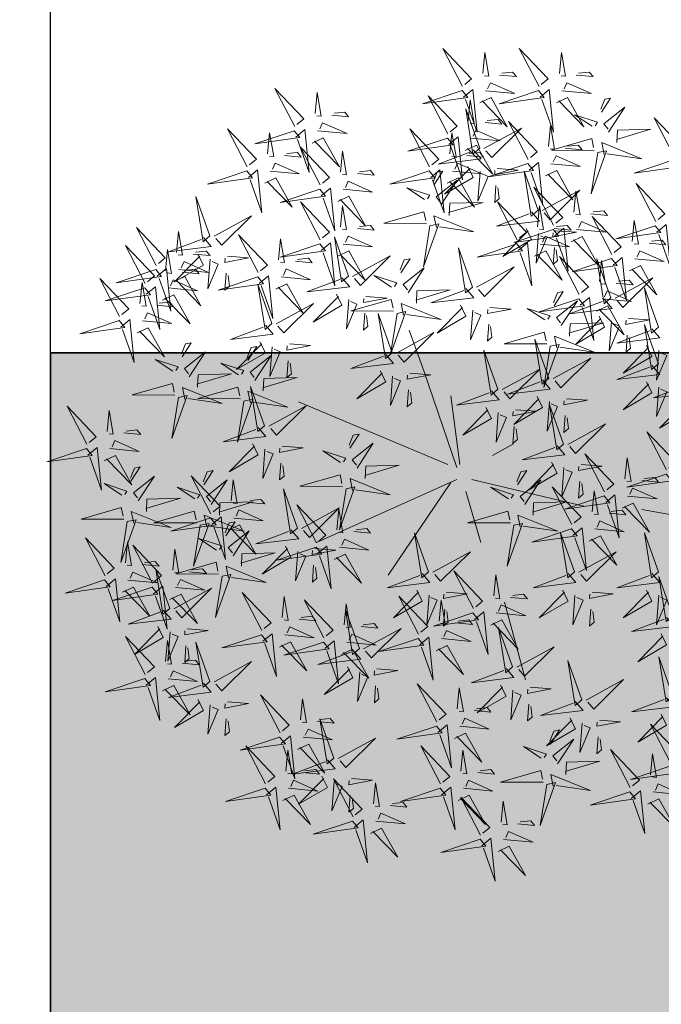
# Model space of a CAD drawing. Units: inches. Extents: x 1704 to 6393, y -157 to 1172.
# Tile 70 of 122: x 1897 to 1920, y 1010 to 1045. Entities that reach past the tile are written whole.
import ezdxf

# ---------------------------------------------------------------- set-up
doc = ezdxf.new("R2010")
doc.units = ezdxf.units.IN
doc.header["$MEASUREMENT"] = 0
for name, color, linetype, lineweight in [('A-ANNO-DIMS', 7, 'Continuous', 13), ('C-PROP', 7, 'Continuous', 35), ('L-shrub', 74, 'Continuous', 18), ('L-tree', 102, 'Continuous', 18)]:
    doc.layers.add(name, color=color, linetype=linetype, lineweight=lineweight)
doc.layers.add('L-HRDS-PATT', color=9, linetype='Continuous', lineweight=13, true_color=0xc5c1ba)
doc.styles.get("Standard").update_dxf_attribs({"font": 'arial.ttf'})
doc.dimstyles.get("Standard").update_dxf_attribs({"dimtxt": 6, "dimasz": 2, "dimexe": 0.18, "dimexo": 0.0625, "dimgap": 0.09, "dimtad": 0, "dimtih": 1, "dimtoh": 1, "dimdec": 1, "dimzin": 0, "dimdsep": 46, "dimlunit": 3, "dimtxsty": 'Standard', "dimblk": 'ARCHTICK', "dimcen": 0.09, "dimadec": 0, "dimazin": 0, "dimtfac": 1, "dimtdec": 1, "dimtofl": 0, "dimtmove": 0, "dimatfit": 3, "dimfxl": 1, "dimtolj": 1, "dimtzin": 0, "dimarcsym": 0})

# ---------------------------------------------------------------- blocks, each defined once
blk = doc.blocks.new('bamboo')
blk.add_line((390, 162.3), (546.4, 218.1))
at = {"layer": 'L-shrub'}
for p, q in [((43.5, 73), (278.2, 631.2)), ((-12.4, 39.5), (-247.1, 564.2)), ((-23.6, 61.9), (-370, 296.3)), ((32.3, 39.5), (390, 162.3)), ((43.5, 28.4), (300.5, 61.9)), ((-57.1, 6), (-247.1, -49.8)), ((-12.4, -16.3), (-113, -440.5)), ((77, -94.4), (121.7, -172.6)), ((-470.6, -139.1), (-761.2, -217.2)), ((-124.2, -652.6), (-157.7, -842.3))]:
    blk.add_line(p, q, dxfattribs=at)
for points in [[(103.7, 1424.7), (54.4, 1572.3), (77.9, 1403.4), (103.7, 1424.7)], [(-387.8, 1356.5), (-437.1, 1504.1), (-413.6, 1335.2), (-387.8, 1356.5)], [(119.4, 1423.2), (261.4, 1496.7), (147.9, 1388.7), (126.6, 1414.5)], [(-160.7, 1284.9), (-160, 1444.8), (-116.9, 1294.1), (-149.7, 1287.2)], [(581.6, 1302), (532.2, 1449.6), (555.7, 1280.7), (581.6, 1302)], [(-372, 1355), (-230.1, 1428.5), (-343.6, 1320.5), (-364.9, 1346.4)], [(79.4, 1419.1), (107.8, 1384.6), (-52.4, 1368.4), (70.8, 1412)], [(597.3, 1300.4), (739.2, 1374), (625.7, 1265.9), (604.4, 1291.8)], [(-756.4, 1206.5), (-805.8, 1354.1), (-782.2, 1185.2), (-756.4, 1206.5)], [(-412.1, 1350.9), (-383.7, 1316.4), (-543.9, 1300.2), (-420.7, 1343.8)], [(-415.1, 1179.2), (-464.4, 1326.8), (-440.9, 1157.9), (-415.1, 1179.2)], [(-70.9, 1292.4), (-27.7, 1358.5), (-55.4, 1272.9), (-68.6, 1281.5)], [(57.7, 1357.7), (77.5, 1316.1), (-31.5, 1255.3), (64.8, 1349.1)], [(103.3, 1337.4), (92.8, 1227.4), (133.3, 1318.7), (110.4, 1328.8)], [(167.7, 1347.1), (246.3, 1339.5), (157.6, 1324.2), (159.1, 1340)], [(704.4, 1206.5), (655.1, 1354.1), (678.6, 1185.2), (704.4, 1206.5)], [(-433.8, 1289.5), (-414, 1248), (-523, 1187.1), (-426.7, 1280.9)], [(-169.3, 1271.7), (-323, 1296.4), (-162.4, 1238.9), (-169.3, 1271.7)], [(557.2, 1296.4), (585.7, 1261.9), (425.4, 1245.7), (548.6, 1289.3)], [(772.7, 1165.6), (723.3, 1313.2), (746.9, 1144.3), (772.7, 1165.6)], [(-740.7, 1205), (-598.8, 1278.5), (-712.2, 1170.5), (-733.6, 1196.4)], [(-500.1, 1137.3), (-534, 1108.2), (-553.5, 1268), (-507.4, 1145.8)], [(-388.2, 1269.3), (-398.7, 1159.2), (-358.2, 1250.5), (-381.1, 1260.6)], [(-323.8, 1278.9), (-245.2, 1271.3), (-333.9, 1256.1), (-332.4, 1271.8)], [(-175.7, 1247.6), (-131.9, 1256.8), (-191.9, 1107.3), (-173.4, 1236.6)], [(-18, 1257.9), (35, 1223.4), (30.4, 1245.3), (-7, 1260.2)], [(161.7, 1284.2), (155.7, 1221.3), (172.9, 1235.5), (168.8, 1275.6)], [(303.5, 1094), (304.2, 1253.9), (347.3, 1103.2), (314.4, 1096.3)], [(720.2, 1205), (862.1, 1278.5), (748.6, 1170.5), (727.3, 1196.4)], [(-561.9, 1157.8), (-603.1, 1137.1), (-666.2, 1244.8), (-570.4, 1150.5)], [(-399.4, 1177.7), (-257.4, 1251.3), (-370.9, 1143.2), (-392.2, 1169.1)], [(-329.8, 1216), (-335.8, 1153.1), (-318.6, 1167.3), (-322.7, 1207.4)], [(-92.2, 1230.9), (0.4, 1170.5), (-61.7, 1248.7), (-81.3, 1233.2)], [(535.5, 1235), (555.3, 1193.4), (446.4, 1132.5), (542.6, 1226.4)], [(581.2, 1214.7), (570.7, 1104.6), (611.1, 1195.9), (588.3, 1206.1)], [(645.6, 1224.3), (724.2, 1216.7), (635.4, 1201.5), (637, 1217.2)], [(788.4, 1164.1), (930.3, 1237.6), (816.9, 1129.6), (795.5, 1155.5)], [(-780.7, 1200.9), (-752.3, 1166.4), (-912.5, 1150.2), (-789.3, 1193.8)], [(-131.4, 1199.8), (-85.3, 1198.1), (-81.9, 1073.4), (-120.4, 1202.1)], [(680.1, 1200.9), (708.6, 1166.4), (548.3, 1150.2), (671.5, 1193.8)], [(-439.4, 1173.7), (-411, 1139.2), (-571.2, 1122.9), (-448, 1166.6)], [(-494, 1113.1), (-347.5, 1165.5), (-515.9, 1138.5), (-494, 1113.1)], [(-174.3, 1012.2), (-173.7, 1172.1), (-130.6, 1021.4), (-163.4, 1014.5)], [(393.3, 1101.5), (436.5, 1167.6), (408.8, 1082), (395.6, 1090.6)], [(748.4, 1160), (776.8, 1125.5), (616.6, 1109.3), (739.8, 1152.9)], [(639.6, 1161.5), (633.5, 1098.6), (650.8, 1112.8), (646.7, 1152.8)], [(-802.5, 1139.6), (-782.6, 1098), (-891.6, 1037.1), (-795.3, 1130.9)], [(-773.2, 987.3), (-807.1, 958.2), (-826.6, 1118), (-780.4, 995.8)], [(-756.8, 1119.3), (-767.3, 1009.2), (-726.8, 1100.5), (-749.7, 1110.6)], [(-692.4, 1128.9), (-613.8, 1121.3), (-702.5, 1106.1), (-701, 1121.8)], [(-581.3, 1111.7), (-691.5, 1120), (-599.4, 1081.4), (-589.8, 1104.4)], [(-461.1, 1112.3), (-441.3, 1070.7), (-550.3, 1009.8), (-454, 1103.7)], [(-155.7, 961.1), (-205, 1108.7), (-181.5, 939.8), (-155.7, 961.1)], [(294.9, 1080.8), (141.2, 1105.5), (301.8, 1048), (294.9, 1080.8)], [(658.4, 1139.6), (678.2, 1098), (569.2, 1037.1), (665.5, 1130.9)], [(704, 1119.3), (693.5, 1009.2), (734, 1100.5), (711.2, 1110.6)], [(768.4, 1128.9), (847.1, 1121.3), (758.3, 1106.1), (759.8, 1121.8)], [(892.5, 987.3), (858.6, 958.2), (839.1, 1118), (885.2, 995.8)], [(-835, 1007.8), (-876.2, 987.1), (-939.2, 1094.8), (-843.4, 1000.5)], [(-495.2, 1097.3), (-418.8, 957), (-529.1, 1068.2), (-503.7, 1090.1)], [(-415.5, 1092), (-426, 981.9), (-385.5, 1073.2), (-408.4, 1083.4)], [(-365.5, 930.4), (-364.8, 1090.2), (-321.7, 939.6), (-354.5, 932.7)], [(-351.1, 1101.6), (-272.5, 1094), (-361.2, 1078.8), (-359.7, 1094.5)], [(-84.5, 1019.7), (-41.3, 1085.8), (-69, 1000.1), (-82.2, 1008.8)], [(446.2, 1067), (499.2, 1032.5), (494.6, 1054.4), (457.2, 1069.3)], [(726.6, 1098.6), (746.5, 1057), (637.5, 996.2), (733.8, 1090)], [(830.7, 1007.8), (789.5, 987.1), (726.4, 1094.8), (822.2, 1000.5)], [(772.3, 1078.4), (761.8, 968.3), (802.3, 1059.6), (779.4, 1069.7)], [(836.7, 1088), (915.3, 1080.4), (826.6, 1065.2), (828.1, 1080.9)], [(-698.4, 1066), (-704.4, 1003.1), (-687.2, 1017.3), (-691.3, 1057.4)], [(-633.3, 1052.3), (-696.3, 1057), (-681.8, 1040.1), (-641.8, 1045)], [(-570.3, 1047.5), (-576.3, 968.8), (-593.4, 1057.2), (-577.6, 1056)], [(-357.1, 1038.7), (-363.1, 975.8), (-345.9, 990), (-350, 1030.1)], [(-140, 959.5), (2, 1033.1), (-111.5, 925), (-132.8, 950.9)], [(288.5, 1056.7), (332.3, 1065.9), (272.3, 916.4), (290.8, 1045.7)], [(372, 1040), (464.6, 979.6), (402.5, 1057.8), (382.9, 1042.3)], [(762.4, 1066), (756.4, 1003.1), (773.6, 1017.3), (769.5, 1057.4)], [(-767.1, 963.1), (-620.5, 1015.5), (-788.9, 988.5), (-767.1, 963.1)], [(-183, 999), (-336.7, 1023.7), (-176.1, 966.2), (-183, 999)], [(-275.7, 937.9), (-232.5, 1004), (-260.1, 918.3), (-273.4, 927)], [(289.9, 848.6), (290.5, 1008.4), (333.6, 857.8), (300.8, 850.9)], [(332.8, 1008.9), (378.9, 1007.2), (382.3, 882.5), (343.8, 1011.2)], [(830.7, 1025.1), (824.7, 962.2), (841.9, 976.4), (837.8, 1016.5)], [(898.5, 963.1), (1045.1, 1015.5), (876.7, 988.5), (898.5, 963.1)], [(-854.3, 961.7), (-964.6, 970), (-872.5, 931.4), (-862.8, 954.4)], [(-189.3, 974.8), (-145.6, 984), (-205.5, 834.6), (-187, 963.9)], [(-105.9, 958.2), (-13.2, 897.8), (-75.4, 976), (-94.9, 960.5)], [(-31.6, 985.2), (21.3, 950.7), (16.7, 972.5), (-20.7, 987.5)], [(811.3, 961.7), (701, 970), (793.1, 931.4), (802.8, 954.4)], [(1141.3, 824.7), (1092, 972.3), (1115.5, 803.4), (1141.3, 824.7)], [(-768.3, 947.3), (-691.9, 807), (-802.2, 918.2), (-776.8, 940.1)], [(-374.1, 917.2), (-527.8, 941.9), (-367.2, 884.4), (-374.1, 917.2)], [(-180, 955.5), (-151.6, 921), (-311.8, 904.8), (-188.6, 948.4)], [(-145, 927.1), (-99, 925.4), (-95.6, 800.6), (-134.1, 929.4)], [(379.6, 856.1), (422.9, 922.2), (395.2, 836.5), (381.9, 845.1)], [(745.4, 783.8), (696, 931.4), (719.6, 762.5), (745.4, 783.8)], [(897.3, 947.3), (973.8, 807), (863.4, 918.2), (888.9, 940.1)], [(-1166, 756.5), (-1215.3, 904.1), (-1191.8, 735.2), (-1166, 756.5)], [(-906.4, 902.3), (-969.4, 907), (-954.8, 890.1), (-914.9, 895)], [(-843.4, 897.5), (-849.4, 818.8), (-866.4, 907.2), (-850.7, 906)], [(-592.6, 770.2), (-641.9, 917.8), (-618.4, 748.9), (-592.6, 770.2)], [(-380.5, 893), (-336.7, 902.2), (-396.6, 752.7), (-378.2, 882.1)], [(-297, 876.4), (-204.4, 816), (-266.5, 894.2), (-286.1, 878.7)], [(-201.7, 894.1), (-181.9, 852.5), (-290.9, 791.6), (-194.6, 885.5)], [(-222.7, 903.4), (-169.8, 868.9), (-174.4, 890.7), (-211.8, 905.7)], [(-91.7, 883.5), (-13.1, 875.8), (-101.8, 860.6), (-100.3, 876.4)], [(120.7, 803.3), (79.5, 782.6), (16.5, 890.3), (112.2, 796)], [(182.5, 782.8), (148.6, 753.6), (129.1, 913.5), (175.2, 791.2)], [(564.8, 755.5), (530.9, 726.4), (511.4, 886.2), (557.5, 764)], [(759.2, 902.3), (696.2, 907), (710.8, 890.1), (750.8, 895)], [(822.2, 897.5), (816.2, 818.8), (799.2, 907.2), (815, 906)], [(1157.1, 823.2), (1299, 896.7), (1185.5, 788.7), (1164.2, 814.6)], [(-974.8, 702), (-1024.2, 849.6), (-1000.7, 680.7), (-974.8, 702)], [(-336.2, 845.3), (-290.1, 843.6), (-286.7, 718.8), (-325.2, 847.6)], [(-156.1, 873.8), (-166.6, 763.7), (-126.1, 855), (-149, 865.2)], [(281.2, 835.4), (127.5, 860.1), (288.1, 802.6), (281.2, 835.4)], [(503, 776), (461.8, 755.3), (398.7, 863), (494.5, 768.7)], [(761.1, 782.3), (903, 855.8), (789.6, 747.8), (768.2, 773.7)], [(-1150.2, 755), (-1008.3, 828.6), (-1121.8, 720.5), (-1143.1, 746.4)], [(-576.8, 768.6), (-434.9, 842.2), (-548.4, 734.1), (-569.7, 760)], [(-97.7, 820.6), (-103.7, 757.7), (-86.5, 771.9), (-90.6, 811.9)], [(188.6, 758.6), (335.2, 810.9), (166.8, 784), (188.6, 758.6)], [(274.9, 811.2), (318.6, 820.4), (258.7, 670.9), (277.2, 800.3)], [(358.3, 794.5), (451, 734.2), (388.8, 812.4), (369.3, 796.8)], [(432.6, 821.6), (485.5, 787.1), (480.9, 808.9), (443.5, 823.9)], [(1117, 819.1), (1145.4, 784.6), (985.2, 768.4), (1108.4, 812)], [(-959.1, 700.5), (-817.2, 774), (-930.7, 666), (-952, 691.8)], [(-199.8, 660.1), (-233.7, 630.9), (-253.2, 790.8), (-207, 668.5)], [(570.9, 731.3), (717.4, 783.7), (549, 756.7), (570.9, 731.3)], [(721.1, 778.2), (749.5, 743.7), (589.3, 727.5), (712.5, 771.1)], [(1291.5, 647.4), (1242.1, 795), (1265.7, 626.1), (1291.5, 647.4)], [(-1190.3, 750.9), (-1161.9, 716.5), (-1322.1, 700.2), (-1198.9, 743.8)], [(-616.9, 764.6), (-588.5, 730.1), (-748.7, 713.9), (-625.5, 757.5)], [(-261.6, 680.5), (-302.7, 659.9), (-365.8, 767.6), (-270, 673.2)], [(101.4, 757.2), (-8.9, 765.5), (83.2, 726.9), (92.9, 749.9)], [(187.4, 742.8), (263.8, 602.4), (153.5, 713.7), (178.9, 735.5)], [(319.2, 763.5), (365.2, 761.8), (368.6, 637), (330.1, 765.8)], [(483.6, 729.9), (373.4, 738.2), (465.5, 699.6), (475.2, 722.6)], [(1095.3, 757.7), (1115.1, 716.2), (1006.1, 655.3), (1102.4, 749.1)], [(1140.9, 737.5), (1130.4, 627.4), (1170.9, 718.7), (1148, 728.8)], [(1205.3, 747.1), (1283.9, 739.5), (1195.2, 724.3), (1196.7, 740)], [(-638.6, 703.2), (-618.8, 661.6), (-727.8, 600.7), (-631.5, 694.6)], [(-264.9, 565.6), (-314.3, 713.2), (-290.7, 544.3), (-264.9, 565.6)], [(49.3, 697.7), (-13.7, 702.5), (0.8, 685.5), (40.8, 690.4)], [(112.3, 693), (106.3, 614.2), (89.3, 702.6), (105, 701.5)], [(569.7, 715.5), (646.1, 575.2), (535.8, 686.4), (561.2, 708.3)], [(699.3, 716.8), (719.2, 675.2), (610.2, 614.4), (706.4, 708.2)], [(809.4, 706.2), (888, 698.6), (799.3, 683.4), (800.8, 699.1)], [(868.3, 552), (818.9, 699.6), (842.4, 530.7), (868.3, 552)], [(1073.1, 552), (1023.7, 699.6), (1047.2, 530.7), (1073.1, 552)], [(1307.2, 645.9), (1449.1, 719.5), (1335.7, 611.4), (1314.3, 637.3)], [(-1212, 689.6), (-1192.2, 648), (-1301.2, 587.1), (-1204.9, 680.9)], [(-1166.4, 669.3), (-1176.9, 559.2), (-1136.4, 650.5), (-1159.3, 660.7)], [(-999.2, 696.4), (-970.7, 661.9), (-1131, 645.7), (-1007.8, 689.3)], [(-1102, 678.9), (-1023.4, 671.3), (-1112.1, 656.1), (-1110.6, 671.8)], [(-619.9, 538.4), (-669.2, 686), (-645.7, 517), (-619.9, 538.4)], [(-593, 682.9), (-603.5, 572.8), (-563, 664.1), (-585.9, 674.3)], [(-528.6, 692.6), (-450, 684.9), (-538.7, 669.7), (-537.2, 685.5)], [(-193.7, 635.8), (-47.1, 688.2), (-215.5, 661.2), (-193.7, 635.8)], [(431.6, 670.5), (368.6, 675.2), (383.1, 658.2), (423.1, 663.2)], [(494.6, 665.7), (488.6, 587), (471.6, 675.4), (487.3, 674.2)], [(745, 696.6), (734.5, 586.5), (774.9, 677.8), (752.1, 687.9)], [(1199.3, 684.2), (1193.3, 621.3), (1210.5, 635.5), (1206.4, 675.6)], [(-1121.7, 544.2), (-1162.9, 523.5), (-1225.9, 631.2), (-1130.2, 536.9)], [(-1059.9, 523.7), (-1093.8, 494.6), (-1113.3, 654.4), (-1067.1, 532.2)], [(-1020.9, 635), (-1001.1, 593.4), (-1110, 532.6), (-1013.8, 626.4)], [(-534.6, 629.7), (-540.6, 566.8), (-523.4, 581), (-527.5, 621)], [(-280.9, 634.5), (-391.2, 642.7), (-299.1, 604.1), (-289.4, 627.2)], [(-249.2, 564.1), (-107.3, 637.7), (-220.7, 529.6), (-242.1, 555.5)], [(-37.8, 466.8), (-37.2, 626.6), (5.9, 476), (-26.9, 469.1)], [(803.4, 643.3), (797.4, 580.4), (814.6, 594.6), (810.5, 634.7)], [(1267.2, 641.9), (1295.6, 607.4), (1135.4, 591.1), (1258.6, 634.8)], [(-1108, 616), (-1114, 553.1), (-1096.8, 567.3), (-1100.9, 607.4)], [(-975.2, 614.7), (-985.8, 504.7), (-945.3, 596), (-968.1, 606.1)], [(-910.8, 624.4), (-832.2, 616.8), (-921, 601.5), (-919.5, 617.3)], [(-604.1, 536.8), (-462.2, 610.4), (-575.7, 502.3), (-597, 528.2)], [(-194.9, 620.1), (-118.4, 479.7), (-228.8, 591), (-203.4, 612.8)], [(742.3, 469.2), (708.4, 440), (688.9, 599.9), (735, 477.6)], [(884, 550.5), (1025.9, 624), (912.4, 516), (891.1, 541.8)], [(1088.8, 550.5), (1230.7, 624), (1117.2, 516), (1095.9, 541.8)], [(-1288.8, 429.3), (-1338.2, 576.9), (-1314.7, 408), (-1288.8, 429.3)], [(-916.9, 561.5), (-922.9, 498.6), (-905.6, 512.8), (-909.7, 552.9)], [(-650.3, 428.2), (-684.2, 399.1), (-703.7, 559), (-657.6, 436.7)], [(-289.2, 560), (-260.8, 525.6), (-421, 509.3), (-297.8, 552.9)], [(-333, 575), (-396, 579.7), (-381.4, 562.8), (-341.5, 567.7)], [(-270, 570.3), (-276, 491.5), (-293, 579.9), (-277.2, 578.7)], [(680.5, 489.6), (639.3, 469), (576.2, 576.7), (672, 482.3)], [(1245.4, 580.5), (1265.3, 538.9), (1156.3, 478), (1252.6, 571.9)], [(1291.1, 560.2), (1280.6, 450.1), (1321.1, 541.4), (1298.2, 551.6)], [(1355.5, 569.8), (1434.1, 562.2), (1345.4, 547), (1346.9, 562.7)], [(-1053.8, 499.5), (-907.2, 551.9), (-1075.6, 524.9), (-1053.8, 499.5)], [(-712.1, 448.7), (-753.3, 428.1), (-816.4, 535.7), (-720.6, 441.4)], [(-644.2, 532.8), (-615.8, 498.3), (-776, 482), (-652.8, 525.7)], [(52, 474.3), (95.2, 540.4), (67.5, 454.7), (54.3, 463.3)], [(843.9, 546.4), (872.4, 511.9), (712.1, 495.7), (835.3, 539.3)], [(1048.7, 546.4), (1077.2, 511.9), (916.9, 495.7), (1040.1, 539.3)], [(-1273.1, 427.7), (-1131.2, 501.3), (-1244.7, 393.3), (-1266, 419.1)], [(-1141, 498.1), (-1251.3, 506.4), (-1159.2, 467.8), (-1149.5, 490.8)], [(-1055, 483.7), (-978.6, 343.4), (-1088.9, 454.6), (-1063.5, 476.4)], [(-311, 498.7), (-291.1, 457.1), (-400.1, 396.2), (-303.9, 490)], [(-200.9, 488), (-122.3, 480.4), (-211, 465.2), (-209.5, 480.9)], [(748.4, 444.9), (894.9, 497.3), (726.5, 470.3), (748.4, 444.9)], [(822.2, 485), (842, 443.4), (733.1, 382.6), (829.3, 476.4)], [(1027, 485), (1046.8, 443.4), (937.9, 382.6), (1034.1, 476.4)], [(1349.5, 506.9), (1343.5, 444), (1360.7, 458.2), (1356.6, 498.3)], [(-1193.1, 438.6), (-1256.1, 443.4), (-1241.5, 426.4), (-1201.6, 431.4)], [(-1130.1, 433.9), (-1136.1, 355.2), (-1153.1, 443.6), (-1137.4, 442.4)], [(-665.9, 471.4), (-646.1, 429.8), (-755.1, 368.9), (-658.8, 462.8)], [(-644.2, 404), (-497.6, 456.4), (-666, 429.4), (-644.2, 404)], [(-620.3, 451.1), (-630.8, 341), (-590.3, 432.3), (-613.2, 442.5)], [(-555.9, 460.7), (-477.3, 453.1), (-566, 437.9), (-564.5, 453.6)], [(-265.3, 478.4), (-275.8, 368.3), (-235.4, 459.6), (-258.2, 469.8)], [(-46.5, 453.6), (-200.1, 478.3), (-39.6, 420.8), (-46.5, 453.6)], [(104.9, 439.8), (157.9, 405.3), (153.3, 427.1), (115.9, 442.1)], [(661.1, 443.6), (550.9, 451.8), (643, 413.2), (652.6, 436.3)], [(867.9, 464.7), (857.4, 354.7), (897.8, 446), (875, 456.1)], [(932.3, 474.4), (1010.9, 466.8), (922.2, 451.6), (923.7, 467.3)], [(1072.7, 464.7), (1062.1, 354.7), (1102.6, 446), (1079.8, 456.1)], [(1137.1, 474.4), (1215.7, 466.8), (1126.9, 451.6), (1128.4, 467.3)], [(-1313.2, 423.7), (-1284.7, 389.2), (-1445, 373), (-1321.8, 416.6)], [(-731.5, 402.7), (-841.7, 410.9), (-749.6, 372.3), (-739.9, 395.4)], [(-206.9, 425.1), (-212.9, 362.2), (-195.7, 376.4), (-199.8, 416.5)], [(-52.8, 429.4), (-9, 438.6), (-69, 289.1), (-50.5, 418.5)], [(30.7, 412.7), (123.3, 352.4), (61.2, 430.6), (41.6, 415)], [(393.8, 326), (352.6, 305.3), (289.5, 413), (385.3, 318.7)], [(455.6, 305.5), (421.7, 276.4), (402.2, 436.3), (448.3, 314)], [(617.5, 275.9), (618.2, 435.7), (661.3, 285.1), (628.5, 278.2)], [(747.2, 429.2), (823.6, 288.8), (713.3, 400), (738.7, 421.9)], [(926.3, 411.5), (920.3, 348.6), (937.5, 362.8), (933.4, 402.9)], [(1131.1, 411.5), (1125, 348.6), (1142.3, 362.8), (1138.2, 402.9)], [(-645.4, 388.3), (-569, 247.9), (-679.3, 359.1), (-653.9, 381)], [(-561.9, 397.8), (-567.9, 334.9), (-550.7, 349.1), (-554.8, 389.2)], [(-8.5, 381.7), (37.5, 380), (40.9, 255.2), (2.4, 384)], [(609.1, 384.1), (546.1, 388.8), (560.6, 371.9), (600.6, 376.8)], [(672.1, 379.4), (666.1, 300.6), (649, 389), (664.8, 387.8)], [(-1334.9, 362.3), (-1315.1, 320.7), (-1424, 259.8), (-1327.8, 353.7)], [(-1289.2, 342), (-1299.8, 231.9), (-1259.3, 323.3), (-1282.1, 333.4)], [(-1224.9, 351.7), (-1146.2, 344), (-1235, 328.8), (-1233.5, 344.6)], [(-783.5, 343.2), (-846.5, 347.9), (-832, 331), (-792, 335.9)], [(-720.5, 338.5), (-726.5, 259.7), (-743.5, 348.1), (-727.8, 346.9)], [(-606.2, 183.8), (-655.6, 331.4), (-632, 162.5), (-606.2, 183.8)], [(461.7, 281.3), (608.2, 333.7), (439.8, 306.7), (461.7, 281.3)], [(707.3, 283.4), (750.5, 349.5), (722.8, 263.8), (709.6, 272.4)], [(-363.6, 169.2), (-397.5, 140), (-417, 299.9), (-370.9, 177.6)], [(945.2, 153.2), (945.8, 313), (988.9, 162.4), (956.1, 155.5)], [(-1230.9, 288.8), (-1236.9, 225.9), (-1219.6, 240.1), (-1223.8, 280.1)], [(-933.9, 115.6), (-983.2, 263.3), (-959.7, 94.3), (-933.9, 115.6)], [(-425.4, 189.6), (-466.6, 169), (-529.7, 276.7), (-433.9, 182.4)], [(374.4, 279.9), (264.1, 288.2), (356.3, 249.6), (365.9, 272.6)], [(460.4, 265.6), (536.9, 125.2), (426.5, 236.4), (452, 258.3)], [(608.9, 262.7), (455.2, 287.4), (615.8, 229.9), (608.9, 262.7)], [(1141.3, 142.9), (1092, 290.5), (1115.5, 121.6), (1141.3, 142.9)], [(-1166, 102), (-1215.3, 249.6), (-1191.8, 80.7), (-1166, 102)], [(-590.5, 182.3), (-448.6, 255.9), (-562, 147.8), (-583.4, 173.7)], [(322.4, 220.5), (259.3, 225.2), (273.9, 208.3), (313.9, 213.2)], [(385.4, 215.7), (379.4, 137), (362.3, 225.4), (378.1, 224.2)], [(602.5, 238.5), (646.3, 247.7), (586.3, 98.2), (604.8, 227.6)], [(686, 221.8), (778.6, 161.5), (716.5, 239.7), (696.9, 224.1)], [(760.2, 248.9), (813.2, 214.4), (808.6, 236.2), (771.2, 251.2)], [(1035, 160.6), (1078.2, 226.8), (1050.5, 141.1), (1037.3, 149.7)], [(1264.2, 74.7), (1214.8, 222.3), (1238.4, 53.4), (1264.2, 74.7)], [(-918.2, 114.1), (-776.2, 187.7), (-889.7, 79.6), (-911, 105.5)], [(-357.5, 145), (-210.9, 197.3), (-379.3, 170.3), (-357.5, 145)], [(646.8, 190.8), (692.9, 189.1), (696.3, 64.3), (657.8, 193.1)], [(1157.1, 141.4), (1299, 214.9), (1185.5, 106.9), (1164.2, 132.8)], [(-1150.2, 100.5), (-1008.3, 174), (-1121.8, 66), (-1143.1, 91.9)], [(-630.5, 178.2), (-602.1, 143.7), (-762.3, 127.5), (-639.2, 171.1)], [(-444.7, 143.6), (-555, 151.8), (-462.9, 113.3), (-453.2, 136.3)], [(936.5, 139.9), (782.9, 164.7), (943.4, 107.2), (936.5, 139.9)], [(1441.7, 20.2), (1392.3, 167.8), (1415.9, -1.1), (1441.7, 20.2)], [(-652.3, 116.9), (-632.5, 75.3), (-741.4, 14.4), (-645.2, 108.2)], [(-510.6, -20.7), (-560, 126.9), (-536.5, -42), (-510.6, -20.7)], [(-358.7, 129.2), (-282.3, -11.2), (-392.6, 100.1), (-367.2, 121.9)], [(639.5, 26), (598.3, 5.3), (535.3, 113), (631, 18.7)], [(701.3, 5.5), (667.4, -23.6), (647.9, 136.3), (694, 14)], [(930.2, 115.8), (973.9, 125), (914, -24.5), (932.5, 104.9)], [(1117, 137.3), (1145.4, 102.8), (985.2, 86.6), (1108.4, 130.2)], [(1013.6, 99.1), (1106.3, 38.8), (1044.2, 116.9), (1024.6, 101.4)], [(1087.9, 126.1), (1140.9, 91.6), (1136.3, 113.5), (1098.9, 128.4)], [(1279.9, 73.2), (1421.8, 146.8), (1308.4, 38.7), (1287, 64.6)], [(-1357.1, -48), (-1406.5, 99.6), (-1382.9, -69.3), (-1357.1, -48)], [(-1190.3, 96.4), (-1161.9, 61.9), (-1322.1, 45.7), (-1198.9, 89.3)], [(-958.2, 110.1), (-929.8, 75.6), (-1090, 59.3), (-966.8, 103)], [(-606.6, 96.6), (-617.1, -13.5), (-576.7, 77.8), (-599.5, 88)], [(-496.8, 84.1), (-559.8, 88.8), (-545.3, 71.9), (-505.3, 76.8)], [(-542.2, 106.2), (-463.6, 98.6), (-552.3, 83.4), (-550.8, 99.1)], [(-433.8, 79.4), (-439.8, 0.6), (-456.8, 89), (-441.1, 87.9)], [(1095.3, 76), (1115.1, 34.4), (1006.1, -26.5), (1102.4, 67.3)], [(1158.3, -1.3), (1117.1, -21.9), (1054.1, 85.8), (1149.8, -8.5)], [(1220.1, -21.7), (1186.2, -50.9), (1166.7, 109), (1212.8, -13.3)], [(1457.4, 18.7), (1599.3, 92.2), (1485.9, -15.8), (1464.5, 10)], [(-979.9, 48.7), (-960.1, 7.1), (-1069.1, -53.8), (-972.8, 40.1)], [(-869.9, 38), (-791.3, 30.4), (-880, 15.2), (-878.5, 30.9)], [(-548.2, 43.3), (-554.2, -19.6), (-537, -5.4), (-541.1, 34.7)], [(-494.9, -22.2), (-353, 51.3), (-466.5, -56.7), (-487.8, -30.9)], [(319, -89.9), (285.1, -119.1), (265.6, 40.8), (311.8, -81.4)], [(974.5, 68.1), (1020.5, 66.3), (1023.9, -58.4), (985.4, 70.4)], [(1239.9, 69.2), (1268.3, 34.7), (1108.1, 18.4), (1231.3, 62.1)], [(1140.9, 55.7), (1130.4, -54.4), (1170.9, 36.9), (1148, 47)], [(1205.3, 65.3), (1283.9, 57.7), (1195.2, 42.5), (1196.7, 58.2)], [(-1341.4, -49.5), (-1199.5, 24), (-1312.9, -84), (-1334.3, -58.1)], [(-1212, 35.1), (-1192.2, -6.5), (-1301.2, -67.4), (-1204.9, 26.4)], [(-1166.4, 14.8), (-1176.9, -95.3), (-1136.4, -4), (-1159.3, 6.1)], [(-1102, 24.4), (-1023.4, 16.8), (-1112.1, 1.6), (-1110.6, 17.3)], [(-934.3, 28.4), (-944.8, -81.7), (-904.3, 9.6), (-927.2, 19.8)], [(257.2, -69.4), (216.1, -90.1), (153, 17.6), (248.8, -76.7)], [(707.4, -18.7), (854, 33.7), (685.6, 6.7), (707.4, -18.7)], [(1218.1, 7.8), (1238, -33.8), (1129, -94.7), (1225.2, -0.8)], [(1199.3, 2.4), (1193.3, -60.5), (1210.5, -46.3), (1206.4, -6.2)], [(1226.2, -46), (1372.8, 6.4), (1204.4, -20.6), (1226.2, -46)], [(1417.4, 14.6), (1445.8, -19.9), (1285.6, -36.1), (1408.7, 7.5)], [(-875.9, -24.9), (-881.9, -87.8), (-864.7, -73.6), (-868.8, -33.5)], [(-718.6, -144.5), (-752.5, -173.6), (-772, -13.7), (-725.8, -136)], [(-535, -26.3), (-506.5, -60.8), (-666.8, -77), (-543.6, -33.4)], [(-174.3, -160.5), (-173.7, -0.6), (-130.6, -151.3), (-163.4, -158.2)], [(620.2, -20.1), (509.9, -11.8), (602, -50.4), (611.7, -27.3)], [(706.2, -34.4), (782.6, -174.8), (672.3, -63.6), (697.7, -41.7)], [(868.3, -184.3), (818.9, -36.7), (842.4, -205.6), (868.3, -184.3)], [(1263.8, -12.5), (1253.3, -122.6), (1293.7, -31.3), (1270.9, -21.1)], [(1328.2, -2.9), (1406.8, -10.5), (1318.1, -25.7), (1319.6, -10)], [(-1381.4, -53.6), (-1353, -88.1), (-1513.2, -104.3), (-1390.1, -60.7)], [(-1108, -38.5), (-1114, -101.4), (-1096.8, -87.2), (-1100.9, -47.1)], [(-780.4, -124), (-821.5, -144.7), (-884.6, -37), (-788.8, -131.3)], [(325.1, -114.1), (471.7, -61.8), (303.3, -88.7), (325.1, -114.1)], [(1139, -47.3), (1028.7, -39.1), (1120.8, -77.6), (1130.5, -54.6)], [(1225, -61.7), (1301.4, -202.1), (1191.1, -90.8), (1216.5, -69)], [(1395.6, -46.8), (1415.5, -88.4), (1306.5, -149.2), (1402.7, -55.4)], [(1322.2, -65.8), (1316.2, -128.7), (1333.4, -114.5), (1329.3, -74.4)], [(1441.3, -67.1), (1430.8, -177.1), (1471.2, -85.8), (1448.4, -75.7)], [(1505.7, -57.4), (1584.3, -65), (1495.6, -80.2), (1497.1, -64.5)], [(-556.7, -87.7), (-536.9, -129.3), (-645.8, -190.1), (-549.6, -96.3)], [(-511, -108), (-521.6, -218), (-481.1, -126.7), (-503.9, -116.6)], [(-446.7, -98.3), (-368, -105.9), (-456.8, -121.2), (-455.3, -105.4)], [(-84.5, -153), (-41.3, -86.9), (-69, -172.5), (-82.2, -163.9)], [(237.9, -115.5), (127.6, -107.2), (219.7, -145.8), (229.4, -122.8)], [(568.1, -79.5), (505.1, -74.8), (519.6, -91.7), (559.6, -86.8)], [(631.1, -84.2), (625.1, -163), (608.1, -74.6), (623.8, -75.8)], [(988, -239.9), (954.1, -269), (934.6, -109.2), (980.8, -231.4)], [(1086.9, -106.8), (1023.9, -102.1), (1038.4, -119), (1078.4, -114.1)], [(1168.6, -225.3), (1119.3, -77.6), (1142.8, -246.6), (1168.6, -225.3)], [(1149.9, -111.5), (1143.9, -190.3), (1126.9, -101.9), (1142.6, -103)], [(-1403.2, -114.9), (-1383.3, -156.5), (-1492.3, -217.4), (-1396.1, -123.6)], [(-1357.5, -135.2), (-1368, -245.3), (-1327.6, -154), (-1350.4, -143.9)], [(-1293.1, -125.6), (-1214.5, -133.2), (-1303.2, -148.4), (-1301.7, -132.7)], [(-1143.7, -283.2), (-1143, -123.3), (-1099.9, -274), (-1132.7, -280.9)], [(-712.5, -168.7), (-565.9, -116.3), (-734.3, -143.3), (-712.5, -168.7)], [(323.9, -129.9), (400.4, -270.3), (290, -159), (315.4, -137.2)], [(494.6, -296.8), (495.3, -137), (538.4, -287.6), (505.6, -294.5)], [(926.2, -219.4), (885, -240.1), (822, -132.4), (917.7, -226.7)], [(884, -185.9), (1025.9, -112.3), (912.4, -220.4), (891.1, -194.5)], [(1441.7, -266.2), (1392.3, -118.6), (1415.9, -287.5), (1441.7, -266.2)], [(1499.7, -120.3), (1493.7, -183.2), (1510.9, -169), (1506.8, -128.9)], [(-799.7, -170.1), (-910, -161.8), (-817.9, -200.4), (-808.2, -177.3)], [(-452.7, -161.2), (-458.7, -224.1), (-441.4, -209.9), (-445.5, -169.8)], [(-183, -173.7), (-336.7, -149), (-176.1, -206.5), (-183, -173.7)], [(185.8, -175), (122.8, -170.2), (137.4, -187.2), (177.4, -182.3)], [(298.2, -260.3), (257, -281), (193.9, -173.3), (289.7, -267.6)], [(248.8, -179.7), (242.8, -258.4), (225.8, -170), (241.6, -171.2)], [(360, -280.8), (326.1, -310), (306.6, -150.1), (352.7, -272.3)], [(922.9, -320.7), (873.5, -173.1), (897.1, -342), (922.9, -320.7)], [(1184.4, -226.8), (1326.3, -153.2), (1212.8, -261.3), (1191.5, -235.4)], [(-1299.1, -188.5), (-1305.1, -251.4), (-1287.9, -237.2), (-1292, -197.1)], [(-1053.9, -275.7), (-1010.7, -209.6), (-1038.4, -295.3), (-1051.6, -286.6)], [(-713.7, -184.4), (-637.3, -324.8), (-747.6, -213.6), (-722.2, -191.7)], [(-189.3, -197.8), (-145.6, -188.6), (-205.5, -338.1), (-187, -208.8)], [(-105.9, -214.5), (-13.2, -274.9), (-75.4, -196.7), (-94.9, -212.2)], [(-31.6, -187.5), (21.3, -222), (16.7, -200.1), (-20.7, -185.2)], [(114.3, -335.4), (80.4, -364.5), (60.9, -204.6), (107, -326.9)], [(843.9, -189.9), (872.4, -224.4), (712.1, -240.6), (835.3, -197)], [(994.1, -264.1), (1140.7, -211.8), (972.3, -238.7), (994.1, -264.1)], [(1457.4, -267.7), (1599.3, -194.1), (1485.9, -302.2), (1464.5, -276.3)], [(-851.8, -229.5), (-914.8, -224.8), (-900.2, -241.7), (-860.3, -236.8)], [(-788.8, -234.2), (-794.8, -313), (-811.8, -224.6), (-796, -225.8)], [(-363.6, -376.3), (-397.5, -405.4), (-417, -245.5), (-370.9, -367.8)], [(-196.6, -388.9), (-246, -241.3), (-222.5, -410.2), (-196.6, -388.9)], [(-145, -245.6), (-99, -247.3), (-95.6, -372), (-134.1, -243.3)], [(52.5, -314.9), (11.3, -335.6), (-51.8, -227.9), (44, -322.2)], [(366.1, -305), (512.7, -252.7), (344.3, -279.6), (366.1, -305)], [(584.4, -289.3), (627.6, -223.2), (600, -308.9), (586.7, -300.3)], [(822.2, -251.3), (842, -292.9), (733.1, -353.8), (829.3, -259.9)], [(906.9, -265.5), (796.6, -257.2), (888.7, -295.8), (898.4, -272.8)], [(938.6, -322.2), (1080.5, -248.7), (967.1, -356.7), (945.7, -330.8)], [(1144.3, -230.8), (1172.7, -265.3), (1012.5, -281.6), (1135.7, -237.9)], [(-1152.3, -296.4), (-1306, -271.7), (-1145.4, -329.2), (-1152.3, -296.4)], [(-841.4, -403.5), (-875.3, -432.7), (-894.8, -272.8), (-848.7, -395.1)], [(-425.4, -355.8), (-466.6, -376.5), (-529.7, -268.8), (-433.9, -363.1)], [(486, -310), (332.3, -285.3), (492.9, -342.8), (486, -310)], [(663.5, -416.2), (614.1, -268.5), (637.6, -437.5), (663.5, -416.2)], [(867.9, -271.6), (857.4, -381.7), (897.8, -290.4), (875, -280.2)], [(932.3, -262), (1010.9, -269.6), (922.2, -284.8), (923.7, -269.1)], [(992.9, -279.9), (1069.3, -420.3), (959, -309), (984.4, -287.2)], [(1122.6, -292.2), (1142.4, -333.8), (1033.4, -394.7), (1129.7, -300.8)], [(1417.4, -271.7), (1445.8, -306.2), (1285.6, -322.5), (1408.7, -278.8)], [(-1158.7, -320.6), (-1114.9, -311.4), (-1174.8, -460.8), (-1156.4, -331.5)], [(-1075.2, -337.2), (-982.6, -397.6), (-1044.7, -319.4), (-1064.3, -334.9)], [(-903.2, -383.1), (-944.4, -403.7), (-1007.5, -296), (-911.7, -390.3)], [(-1000.9, -310.2), (-948, -344.7), (-952.6, -322.9), (-990, -307.9)], [(-180.9, -390.4), (-39, -316.9), (-152.5, -424.9), (-173.8, -399)], [(120.3, -359.6), (266.9, -307.2), (98.5, -334.2), (120.3, -359.6)], [(278.8, -306.4), (168.6, -298.1), (260.7, -336.7), (270.4, -313.7)], [(364.9, -320.8), (441.3, -461.2), (331, -349.9), (356.4, -328.1)], [(479.7, -334.2), (523.4, -325), (463.5, -474.5), (482, -345.1)], [(637.4, -323.8), (690.3, -358.3), (685.7, -336.5), (648.3, -321.5)], [(898.6, -326.3), (927, -360.8), (766.8, -377), (889.9, -333.4)], [(854.8, -325), (791.8, -320.2), (806.4, -337.2), (846.3, -332.2)], [(917.8, -329.7), (911.8, -408.4), (894.8, -320), (910.5, -321.2)], [(926.3, -324.9), (920.3, -387.8), (937.5, -373.5), (933.4, -333.5)], [(1168.2, -312.5), (1157.7, -422.6), (1198.2, -331.3), (1175.3, -321.1)], [(1218.2, -474.1), (1218.9, -314.2), (1262, -464.9), (1229.2, -471.8)], [(1232.6, -302.9), (1311.2, -310.5), (1222.5, -325.7), (1224, -310)], [(-1114.4, -368.3), (-1068.3, -370), (-1064.9, -494.8), (-1103.4, -366)], [(-357.5, -400.5), (-210.9, -348.1), (-379.3, -375.1), (-357.5, -400.5)], [(-73.8, -511.6), (-123.1, -364), (-99.6, -532.9), (-73.8, -511.6)], [(33.1, -361), (-77.2, -352.7), (14.9, -391.3), (24.6, -368.2)], [(226.8, -365.9), (163.8, -361.1), (178.3, -378.1), (218.3, -373.2)], [(289.8, -370.6), (283.8, -449.3), (266.8, -360.9), (282.5, -362.1)], [(563.1, -350.9), (655.8, -411.2), (593.6, -333), (574, -348.6)], [(679.2, -417.7), (821.1, -344.1), (707.7, -452.2), (686.3, -426.3)], [(1226.6, -365.8), (1220.6, -428.7), (1237.8, -414.5), (1233.7, -374.4)], [(1395.6, -333.1), (1415.5, -374.7), (1306.5, -435.6), (1402.7, -341.7)], [(1441.3, -353.4), (1430.8, -463.5), (1471.2, -372.2), (1448.4, -362)], [(1505.7, -343.8), (1584.3, -351.4), (1495.6, -366.6), (1497.1, -350.9)], [(-835.4, -427.8), (-688.8, -375.4), (-857.2, -402.4), (-835.4, -427.8)], [(-444.7, -401.9), (-555, -393.6), (-462.9, -432.2), (-453.2, -409.1)], [(-221, -394.5), (-192.5, -429), (-352.8, -445.2), (-229.6, -401.6)], [(119.1, -375.3), (195.6, -515.7), (85.2, -404.5), (110.7, -382.6)], [(524, -381.9), (570, -383.6), (573.4, -508.4), (534.9, -379.6)], [(660.4, -512.6), (626.5, -541.8), (607, -381.9), (653.1, -504.2)], [(813.7, -538.9), (764.3, -391.3), (787.8, -560.2), (813.7, -538.9)], [(876.8, -387.7), (896.6, -429.3), (787.7, -490.1), (883.9, -396.3)], [(986.9, -398.3), (1065.5, -405.9), (976.8, -421.1), (978.3, -405.4)], [(1308, -466.6), (1351.2, -400.5), (1323.6, -486.2), (1310.3, -477.5)], [(-922.6, -429.1), (-1032.9, -420.9), (-940.7, -459.5), (-931.1, -436.4)], [(-358.7, -416.2), (-282.3, -556.6), (-392.6, -445.4), (-367.2, -423.5)], [(-19, -420.4), (-82, -415.7), (-67.4, -432.6), (-27.4, -427.7)], [(-58, -513.1), (83.9, -439.6), (-29.6, -547.6), (-50.9, -521.7)], [(44, -425.1), (38, -503.9), (21, -415.5), (36.8, -416.7)], [(598.6, -492.1), (557.4, -512.8), (494.3, -405.1), (590.1, -499.4)], [(639.2, -421.7), (667.6, -456.2), (507.4, -472.5), (630.5, -428.8)], [(922.5, -407.9), (912, -518), (952.4, -426.7), (929.6, -416.6)], [(1499.7, -406.7), (1493.7, -469.6), (1510.9, -455.4), (1506.8, -415.3)], [(-1179.6, -607.1), (-1229, -459.4), (-1205.5, -628.4), (-1179.6, -607.1)], [(-836.6, -443.5), (-760.1, -583.9), (-870.5, -472.6), (-845, -450.8)], [(-496.8, -461.3), (-559.8, -456.6), (-545.3, -473.5), (-505.3, -468.6)], [(-433.8, -466), (-439.8, -544.8), (-456.8, -456.4), (-441.1, -457.6)], [(-242.7, -455.8), (-222.9, -497.4), (-331.8, -558.3), (-235.6, -464.5)], [(-197, -476.1), (-207.5, -586.2), (-167.1, -494.9), (-189.9, -484.8)], [(-132.6, -466.5), (-54, -474.1), (-142.8, -489.3), (-141.3, -473.6)], [(829.4, -540.4), (971.3, -466.8), (857.8, -574.9), (836.5, -549)], [(980.9, -461.2), (974.9, -524.1), (992.1, -509.9), (988, -469.8)], [(1209.6, -487.3), (1055.9, -462.6), (1216.5, -520.1), (1209.6, -487.3)], [(-974.6, -488.6), (-1037.7, -483.9), (-1023.1, -500.8), (-983.1, -495.9)], [(-911.6, -493.3), (-917.6, -572.1), (-934.7, -483.7), (-918.9, -484.8)], [(617.4, -483.1), (637.2, -524.7), (528.3, -585.6), (624.5, -491.7)], [(666.4, -536.8), (813, -484.5), (644.6, -511.4), (666.4, -536.8)], [(663.1, -503.4), (652.6, -613.5), (693, -522.2), (670.2, -512)], [(727.5, -493.8), (806.1, -501.4), (717.4, -516.6), (718.9, -500.9)], [(1203.3, -511.5), (1247, -502.3), (1187.1, -651.7), (1205.5, -522.4)], [(1286.7, -528.1), (1379.3, -588.5), (1317.2, -510.3), (1297.6, -525.8)], [(1361, -501.1), (1413.9, -535.6), (1409.3, -513.8), (1371.9, -498.8)], [(-1163.9, -608.6), (-1022, -535), (-1135.5, -643.1), (-1156.8, -617.2)], [(-98.1, -517.2), (-69.7, -551.7), (-229.9, -567.9), (-106.7, -524.3)], [(-138.6, -529.4), (-144.7, -592.3), (-127.4, -578.1), (-131.5, -538)], [(579.2, -538.2), (468.9, -529.9), (561.1, -568.5), (570.7, -545.5)], [(789.3, -544.5), (817.8, -578.9), (657.5, -595.2), (780.7, -551.6)], [(-425.4, -669.4), (-466.6, -690.1), (-529.7, -582.4), (-433.9, -676.7)], [(-363.6, -689.9), (-397.5, -719), (-417, -559.2), (-370.9, -681.4)], [(-119.8, -578.6), (-100, -620.2), (-209, -681), (-112.7, -587.2)], [(352.8, -669.4), (311.6, -690.1), (248.5, -582.4), (344.3, -676.7)], [(414.6, -689.9), (380.7, -719), (361.2, -559.2), (407.3, -681.4)], [(489.3, -669.4), (448.2, -690.1), (385.1, -582.4), (480.9, -676.7)], [(551.1, -689.9), (517.2, -719), (497.7, -559.2), (543.9, -681.4)], [(665.2, -552.6), (741.7, -693), (631.3, -581.7), (656.8, -559.9)], [(721.5, -556.7), (715.5, -619.6), (732.7, -605.4), (728.6, -565.3)], [(936.5, -702.5), (887.2, -554.9), (910.7, -723.8), (936.5, -702.5)], [(1247.5, -559.2), (1293.6, -560.9), (1297, -685.7), (1258.5, -556.9)], [(-1204, -612.6), (-1175.5, -647.1), (-1335.8, -663.4), (-1212.6, -619.7)], [(-1084.1, -757), (-1133.4, -609.4), (-1109.9, -778.4), (-1084.1, -757)], [(-827.8, -744.4), (-861.7, -773.6), (-881.2, -613.7), (-835.1, -736)], [(-527.4, -744.4), (-561.3, -773.6), (-580.8, -613.7), (-534.7, -736)], [(-74.2, -598.9), (-84.7, -708.9), (-44.2, -617.6), (-67, -607.5)], [(8.2, -743.4), (-41.2, -595.8), (-17.7, -764.7), (8.2, -743.4)], [(-9.8, -589.2), (68.8, -596.8), (-19.9, -612), (-18.4, -596.3)], [(527.1, -597.7), (464.1, -593), (478.7, -609.9), (518.7, -605)], [(590.2, -602.4), (584.1, -681.2), (567.1, -592.8), (582.9, -593.9)], [(767.6, -605.8), (787.4, -647.4), (678.5, -708.3), (774.7, -614.5)], [(877.7, -616.5), (956.3, -624.1), (867.5, -639.3), (869, -623.6)], [(1182.3, -770.7), (1132.9, -623.1), (1156.5, -792), (1182.3, -770.7)], [(-889.6, -724), (-930.8, -744.6), (-993.8, -636.9), (-898.1, -731.2)], [(-589.2, -724), (-630.4, -744.6), (-693.5, -636.9), (-597.7, -731.2)], [(-357.5, -714.1), (-210.9, -661.7), (-379.3, -688.7), (-357.5, -714.1)], [(-15.8, -652.1), (-21.8, -715), (-4.6, -700.8), (-8.7, -660.7)], [(420.7, -714.1), (567.3, -661.7), (398.9, -688.7), (420.7, -714.1)], [(557.2, -714.1), (703.8, -661.7), (535.4, -688.7), (557.2, -714.1)], [(813.3, -626.1), (802.7, -736.2), (843.2, -644.9), (820.4, -634.7)], [(952.3, -704), (1094.2, -630.5), (980.7, -738.5), (959.4, -712.7)], [(-1225.7, -674), (-1205.9, -715.6), (-1314.8, -776.5), (-1218.6, -682.6)], [(-1180, -694.3), (-1190.5, -804.4), (-1150.1, -713.1), (-1172.9, -702.9)], [(-1115.6, -684.7), (-1037, -692.3), (-1125.7, -707.5), (-1124.2, -691.8)], [(-1068.3, -758.6), (-926.4, -685), (-1039.9, -793.1), (-1061.2, -767.2)], [(23.9, -744.9), (165.8, -671.4), (52.3, -779.4), (31, -753.6)], [(346.4, -826.2), (312.4, -855.4), (293, -695.5), (339.1, -817.8)], [(871.6, -679.4), (865.6, -742.3), (882.9, -728.1), (878.8, -688)], [(1198, -772.2), (1339.9, -698.7), (1226.5, -806.7), (1205.1, -780.8)], [(-821.7, -768.6), (-675.1, -716.3), (-843.5, -743.3), (-821.7, -768.6)], [(-444.7, -715.5), (-555, -707.2), (-462.9, -745.8), (-453.2, -722.8)], [(-521.3, -768.6), (-374.8, -716.3), (-543.2, -743.3), (-521.3, -768.6)], [(284.5, -805.8), (243.4, -826.4), (180.3, -718.7), (276.1, -813.1)], [(333.5, -715.5), (223.2, -707.2), (315.3, -745.8), (325, -722.8)], [(470, -715.5), (359.7, -707.2), (451.8, -745.8), (461.5, -722.8)], [(912.2, -708.1), (940.6, -742.6), (780.4, -758.8), (903.6, -715.2)]]:
    blk.add_lwpolyline(points, dxfattribs=at)
blk = doc.blocks.new('_ArchTick')
at = {"color": 0, "linetype": 'ByBlock', "const_width": 0.15}
blk.add_lwpolyline([(-0.5, -0.5), (0.5, 0.5)], dxfattribs=at)
blk = doc.blocks.new('*D94')
at = {"layer": 'A-ANNO-DIMS', "color": 0, "lineweight": -2, "transparency": 16777216}
for p, q in [((1898.349, 895.275), (1898.349, 1105.287)), ((1898.349, 1105.107), (1979.39, 1105.107)), ((2073.349, 1105.107), (1992.307, 1105.107)), ((2073.349, 895.275), (2073.349, 1105.287))]:
    blk.add_line(p, q, dxfattribs=at)
at = {"layer": 'Defpoints', "color": 0, "lineweight": -3, "transparency": 16777216}
for p in [(2073.349, 1105.107), (1898.349, 895.213), (2073.349, 895.213)]:
    blk.add_point(p, dxfattribs=at)
at = {"layer": 'A-ANNO-DIMS', "color": 0, "lineweight": -2, "transparency": 16777216, "xscale": 2, "yscale": 2, "zscale": 2, "rotation": 180}
blk.add_blockref('_ArchTick', (1898.349, 1105.107), dxfattribs=at)
at = {"layer": 'A-ANNO-DIMS', "color": 0, "lineweight": -2, "transparency": 16777216, "xscale": 2, "yscale": 2, "zscale": 2}
blk.add_blockref('_ArchTick', (2073.349, 1105.107), dxfattribs=at)
at = {"layer": 'A-ANNO-DIMS', "color": 0, "transparency": 16777216, "insert": (1985.849, 1105.107), "char_height": 6, "attachment_point": 5}
blk.add_mtext('\\A1;175', dxfattribs=at)

msp = doc.modelspace()

# ---------------------------------------------------------------- hatches: boundary and pattern name
at = {"layer": 'L-HRDS-PATT', "transparency": 33554643}
h = msp.add_hatch(color=256, dxfattribs=at)
h.dxf.hatch_style = 1
h.paths.add_polyline_path([(2065.589, 1033.213), (1898.349, 1033.213), (1898.349, 895.213), (2065.589, 895.213)])

# ---------------------------------------------------------------- linework, layer by layer
at = {"layer": 'C-PROP'}
for p in [(1898.349, -3.787), (2723.349, 1033.213)]:
    msp.add_line(p, (1898.349, 1033.213), dxfattribs=at)

# ---------------------------------------------------------------- block references
at = {"layer": 'L-tree', "xscale": 0.0095734028514679, "yscale": 0.0095734028514679, "zscale": 0.0095734028514679, "rotation": 89.99999999999996}
msp.add_blockref('bamboo', (1913.269, 1028.796), dxfattribs=at)

# ---------------------------------------------------------------- dimensions: what is measured, and where the dimension line sits
at = {"layer": 'A-ANNO-DIMS'}
dim = msp.add_linear_dim(base=(2073.349, 1105.107), p1=(1898.349, 895.213), p2=(2073.349, 895.213), dimstyle='Standard', override={"dimdec": 0, "dimlfac": 1, "dimrnd": 0, "dimzin": 0, "dimdsep": 46, "dimlunit": 2}, dxfattribs=at)
dim.commit()
dim.dimension.update_dxf_attribs({"geometry": '*D94', "text_midpoint": (1985.849, 1105.107)})

doc.saveas('drawing.dxf')
